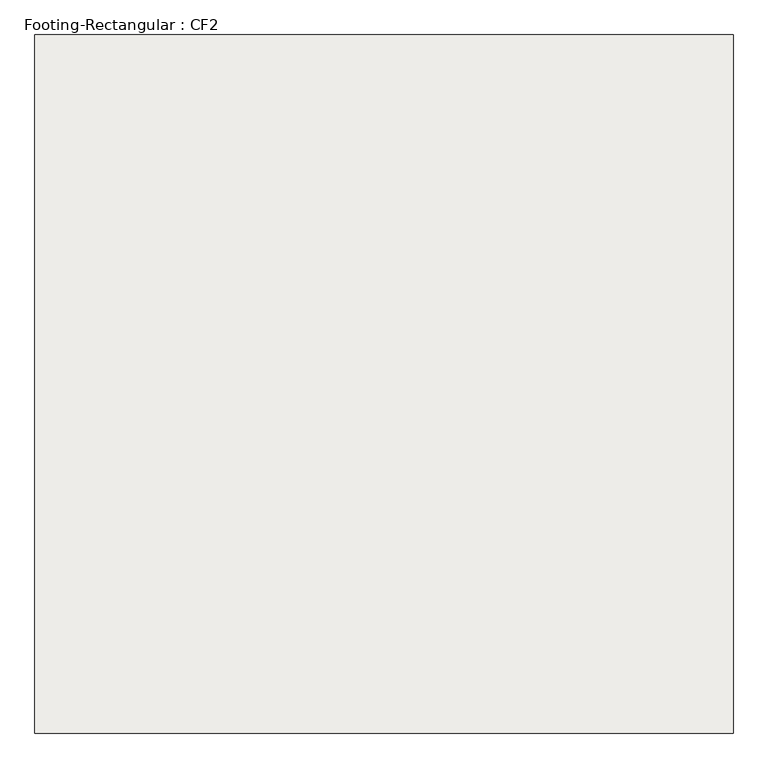
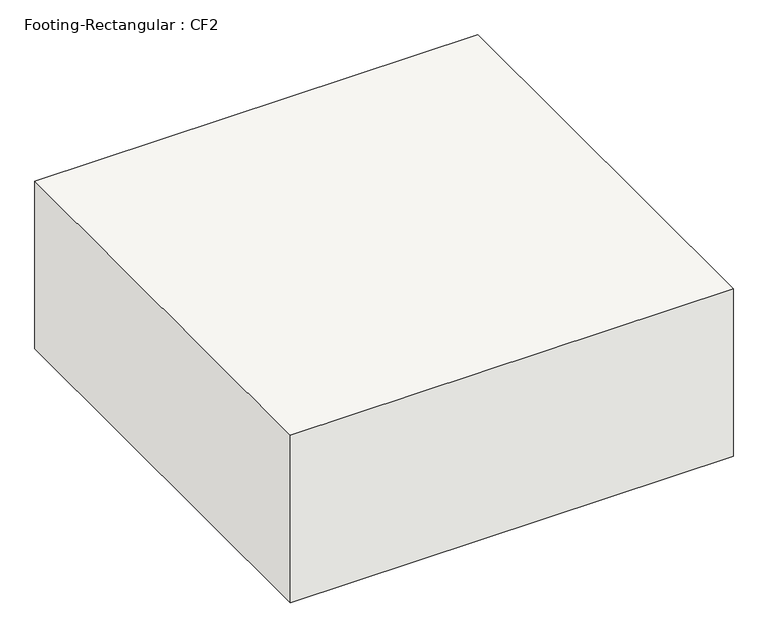
"""IFC4 building model written with IfcOpenShell, lengths in millimetres: slab geometry, Footing-Rectangular : CF2."""

from ifc_helpers import new_model, si_unit, frame, origin, place, context, project, spatial, polyline, outline, extrude, source, transform, mapped, element, save


def footing_rectangular_cf2_90c2f4b8(model_context):
    return source(origin(), model_context, "Body", "SweptSolid", [
        extrude(outline(polyline([(571.5, 571.5), (571.5, -571.5), (-571.5, -571.5), (-571.5, 571.5), (571.5, 571.5)])), frame((0.0, 0.0, -457.2), z_axis=(0.0, 0.0, 1.0), x_axis=(1.0, 0.0, 0.0)), (0.0, 0.0, 1.0), 457.2),
    ])


if __name__ == "__main__":
    model = new_model("IFC4")
    model_context = context("Model", 3, world=origin())
    ifc_project = project(units=[si_unit("LENGTHUNIT", "METRE", prefix="MILLI")], contexts=[model_context])
    site = spatial("IfcSite", under=ifc_project)
    building = spatial("IfcBuilding", under=site)
    placement = place(None, origin())
    footing_rectangular_cf2_shape = footing_rectangular_cf2_90c2f4b8(model_context)
    element("IfcSlab", 1, ObjectType="Footing-Rectangular : CF2", at=placement, inside=building, context=model_context, shape_type="MappedRepresentation", body=[
        mapped(footing_rectangular_cf2_shape, transform((0.0, 0.0, 0.0), x_axis=(1.0, 0.0, 0.0), y_axis=(0.0, 1.0, 0.0), z_axis=(0.0, 0.0, 1.0))),
    ])
    save(model, "model.ifc")

# Revit data of these elements
# Type "Footing-Rectangular : CF2"
#   Width = 1143 mm
#   Length = 1143 mm
#   Foundation Thickness = 457.2 mm
#   Structural Material [instance default] = Concrete - Cast-in-Place Concrete
#   Assembly Code = ""
# Element 1 (IfcSlab, "Footing-Rectangular : CF2")
#   Materials on its faces: "Concrete - Cast-in-Place Concrete"
# Materials
#   "Concrete - Cast-in-Place Concrete": class "Concrete", colour RGB 192 192 192, transparency 0, Cost = 0
